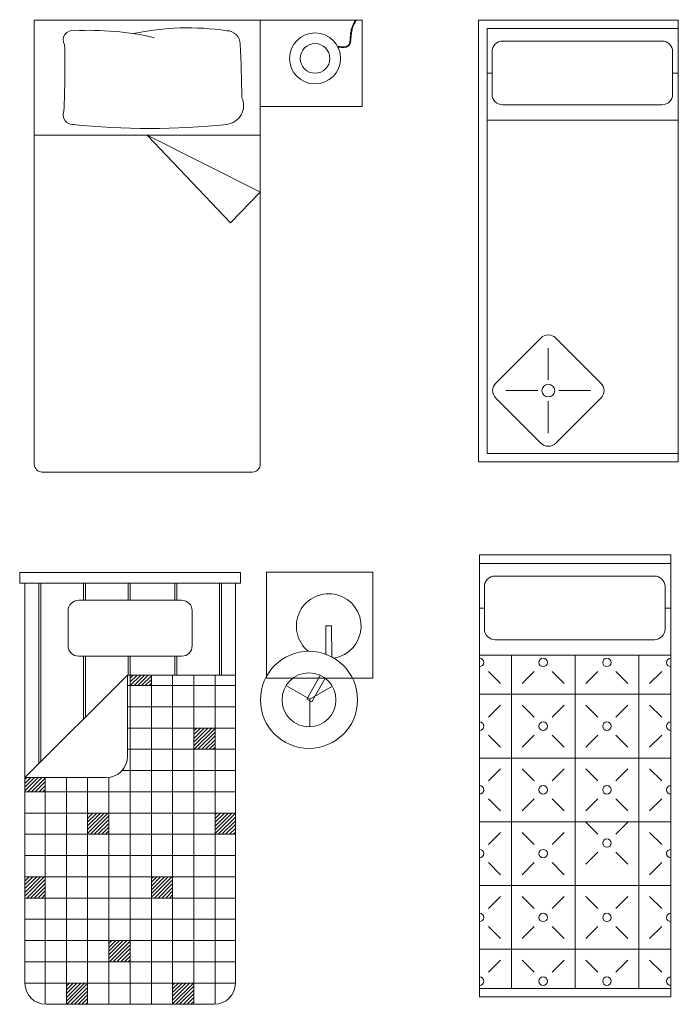
# Model space of a CAD drawing. Units: inches. Extents: x 1994 to 3075, y 3517 to 3950.
# Tile 3 of 58: x 1993.7652 to 1993.8873, y 3553.3272 to 3553.5096. Entities that reach past the tile are written whole.
import ezdxf

# ---------------------------------------------------------------- set-up
doc = ezdxf.new("R2010")
doc.units = ezdxf.units.IN
doc.layers.add('A-FURN-REFR', color=8, linetype='Continuous', lineweight=13)
doc.layers.add('A-FURN-REFR-PATT', color=8, linetype='Continuous', lineweight=13)
pattern_1 = [(45, (0, 0), (-0.0003479856204649, 0.0003479856204649), [])]
pattern_2 = [(45, (0, 0), (-0.0003479856200101, 0.0003479856200101), [])]

msp = doc.modelspace()

# ---------------------------------------------------------------- hatches: boundary and pattern name
at = {"layer": 'A-FURN-REFR-PATT'}
h = msp.add_hatch(dxfattribs=at)
h.set_pattern_fill('ANSI31', color=256, scale=0.00015500030971, style=0)
h.set_pattern_definition(pattern_2)
h.paths.add_polyline_path([(1993.785672265221, 3553.3862541341), (1993.789609273095, 3553.3862541341), (1993.789609273095, 3553.388199015989), (1993.785672265221, 3553.388199015989)])
h = msp.add_hatch(dxfattribs=at)
h.set_pattern_fill('ANSI31', color=256, scale=0.0001550003099125, style=0)
h.set_pattern_definition(pattern_1)
h.paths.add_polyline_path([(1993.797483288843, 3553.374443110477), (1993.801420296717, 3553.374443110477), (1993.801420296717, 3553.37838011835), (1993.797483288843, 3553.37838011835)])
h = msp.add_hatch(dxfattribs=at)
h.set_pattern_fill('ANSI31', color=256, scale=0.0001550003099125, style=0)
h.set_pattern_definition(pattern_1)
h.paths.add_polyline_path([(1993.766172265221, 3553.366569094728), (1993.769924233725, 3553.366569094728), (1993.769924233725, 3553.369199015988), (1993.766172265221, 3553.369199015988)])
h = msp.add_hatch(dxfattribs=at)
h.set_pattern_fill('ANSI31', color=256, scale=0.0001550003099125, style=0)
h.set_pattern_definition(pattern_1)
h.paths.add_polyline_path([(1993.777798249473, 3553.35869507898), (1993.781735257347, 3553.35869507898), (1993.781735257347, 3553.362632086854), (1993.777798249473, 3553.362632086854)])
h = msp.add_hatch(dxfattribs=at)
h.set_pattern_fill('ANSI31', color=256, scale=0.0001550003099125, style=0)
h.set_pattern_definition(pattern_1)
h.paths.add_polyline_path([(1993.801420296717, 3553.35869507898), (1993.805172265221, 3553.35869507898), (1993.805172265221, 3553.362632086854), (1993.801420296717, 3553.362632086854)])
h = msp.add_hatch(dxfattribs=at)
h.set_pattern_fill('ANSI31', color=256, scale=0.0001550003099125, style=0)
h.set_pattern_definition(pattern_1)
h.paths.add_polyline_path([(1993.766172265221, 3553.346884055358), (1993.769924233725, 3553.346884055358), (1993.769924233725, 3553.350821063232), (1993.766172265221, 3553.350821063232)])
h = msp.add_hatch(dxfattribs=at)
h.set_pattern_fill('ANSI31', color=256, scale=0.0001550003099125, style=0)
h.set_pattern_definition(pattern_1)
h.paths.add_polyline_path([(1993.789609273095, 3553.346884055358), (1993.793546280969, 3553.346884055358), (1993.793546280969, 3553.350821063232), (1993.789609273095, 3553.350821063232)])
h = msp.add_hatch(dxfattribs=at)
h.set_pattern_fill('ANSI31', color=256, scale=0.0001550003099125, style=0)
h.set_pattern_definition(pattern_1)
h.paths.add_polyline_path([(1993.781735257347, 3553.335073031736), (1993.785672265221, 3553.335073031736), (1993.785672265221, 3553.339010039611), (1993.781735257347, 3553.339010039611)])
h = msp.add_hatch(dxfattribs=at)
h.set_pattern_fill('ANSI31', color=256, scale=0.0001550003099125, style=0)
h.set_pattern_definition(pattern_1)
h.paths.add_polyline_path([(1993.773861241599, 3553.327199015988), (1993.777798249473, 3553.327199015988), (1993.777798249473, 3553.331136023862), (1993.773861241599, 3553.331136023862)])
h = msp.add_hatch(dxfattribs=at)
h.set_pattern_fill('ANSI31', color=256, scale=0.00015500030971, style=0)
h.set_pattern_definition(pattern_2)
h.paths.add_polyline_path([(1993.793546280969, 3553.327199015988), (1993.797483288843, 3553.327199015988), (1993.797483288843, 3553.331136023862), (1993.793546280969, 3553.331136023862)])

# ---------------------------------------------------------------- linework, layer by layer
at = {"layer": 'A-FURN-REFR'}
for p, q in [((1993.809793398791, 3553.509573136487), (1993.767915594969, 3553.509573136487)), ((1993.809793398791, 3553.509573136487), (1993.767915594969, 3553.509573136487)), ((1993.767915594969, 3553.509573136487), (1993.767915594969, 3553.427281987548)), ((1993.767915594969, 3553.488246379321), (1993.767915594969, 3553.509573136487)), ((1993.767915594969, 3553.509573136487), (1993.809793398791, 3553.509573136487)), ((1993.809793398791, 3553.509573136487), (1993.767915594969, 3553.509573136487)), ((1993.809793398791, 3553.509573136487), (1993.767915594969, 3553.509573136487)), ((1993.767915594969, 3553.509573136487), (1993.767915594969, 3553.427281987548)), ((1993.767915594969, 3553.488246379321), (1993.767915594969, 3553.509573136487)), ((1993.767915594969, 3553.509573136487), (1993.809793398791, 3553.509573136487)), ((1993.809793398791, 3553.509573136487), (1993.828638410511, 3553.509573136487)), ((1993.809793398791, 3553.49355757055), (1993.809793398791, 3553.509573136487)), ((1993.809793398791, 3553.509573136487), (1993.828638410511, 3553.509573136487)), ((1993.809793398791, 3553.509573136487), (1993.809793398791, 3553.488246379321)), ((1993.809793398791, 3553.509573136487), (1993.828638410511, 3553.509573136487)), ((1993.809793398791, 3553.49355757055), (1993.809793398791, 3553.509573136487)), ((1993.809793398791, 3553.509573136487), (1993.828638410511, 3553.509573136487)), ((1993.809793398791, 3553.509573136487), (1993.809793398791, 3553.488246379321)), ((1993.828638410511, 3553.509573136487), (1993.828638410511, 3553.49355757055)), ((1993.828638410511, 3553.509573136487), (1993.828638410511, 3553.49355757055)), ((1993.828638410511, 3553.509573136487), (1993.828638410511, 3553.49355757055)), ((1993.828638410511, 3553.509573136487), (1993.828638410511, 3553.49355757055)), ((1993.850243684991, 3553.427685512103), (1993.850243684991, 3553.509575275882)), ((1993.887251559007, 3553.509575275882), (1993.850243684991, 3553.509575275882)), ((1993.887251559007, 3553.427685512103), (1993.887251559007, 3553.509575275882)), ((1993.85181848814, 3553.429260315252), (1993.85181848814, 3553.508000472733)), ((1993.887251559007, 3553.508000472733), (1993.85181848814, 3553.508000472733)), ((1993.884228804072, 3553.50566943182), (1993.854701245017, 3553.50566943182)), ((1993.85273274108, 3553.503700927882), (1993.85273274108, 3553.495826912135)), ((1993.886197308009, 3553.495826912135), (1993.886197308009, 3553.503700927882)), ((1993.85181848814, 3553.499707984479), (1993.85273274108, 3553.499707984479)), ((1993.886197308009, 3553.499707984479), (1993.887251559007, 3553.499707984479)), ((1993.828638410511, 3553.49355757055), (1993.809793398791, 3553.49355757055)), ((1993.828638410511, 3553.49355757055), (1993.809793398791, 3553.49355757055)), ((1993.809793398791, 3553.427281987548), (1993.809793398791, 3553.49355757055)), ((1993.828638410511, 3553.49355757055), (1993.809793398791, 3553.49355757055)), ((1993.828638410511, 3553.49355757055), (1993.809793398791, 3553.49355757055)), ((1993.809793398791, 3553.427281987548), (1993.809793398791, 3553.49355757055)), ((1993.854701245017, 3553.493858408198), (1993.884228804072, 3553.493858408198)), ((1993.887251559007, 3553.491004982646), (1993.85181848814, 3553.491004982646)), ((1993.78885449688, 3553.488246379321), (1993.767915594969, 3553.488246379321)), ((1993.809793398791, 3553.488246379321), (1993.767915594969, 3553.488246379321)), ((1993.78885449688, 3553.488246379321), (1993.767915594969, 3553.488246379321)), ((1993.809793398791, 3553.488246379321), (1993.767915594969, 3553.488246379321)), ((1993.78885449688, 3553.488246379321), (1993.809804655327, 3553.477674335062)), ((1993.78885449688, 3553.488246379321), (1993.804276123482, 3553.472010531263)), ((1993.78885449688, 3553.488246379321), (1993.809804655327, 3553.477674335062)), ((1993.78885449688, 3553.488246379321), (1993.804276123482, 3553.472010531263)), ((1993.804276123482, 3553.472013370684), (1993.809793398791, 3553.477680015429)), ((1993.804276123482, 3553.472013370684), (1993.809793398791, 3553.477680015429)), ((1993.861770166646, 3553.450651259108), (1993.853418511751, 3553.442299604212)), ((1993.872905706508, 3553.442299604212), (1993.864554051612, 3553.450651259108)), ((1993.863162109129, 3553.448781677478), (1993.863162109129, 3553.442876165667)), ((1993.855288093381, 3553.440907661729), (1993.861193605192, 3553.440907661729)), ((1993.865130613066, 3553.440907661729), (1993.871036124877, 3553.440907661729)), ((1993.853418511751, 3553.439515719247), (1993.861770166646, 3553.431164064351)), ((1993.863162109129, 3553.438939157793), (1993.863162109129, 3553.433033645982)), ((1993.864554051612, 3553.431164064351), (1993.872905706508, 3553.439515719247)), ((1993.85181848814, 3553.429260315252), (1993.887251559007, 3553.429260315252)), ((1993.850243684991, 3553.427685512103), (1993.887251559007, 3553.427685512103)), ((1993.769380053673, 3553.425817528844), (1993.808328940087, 3553.425817528844)), ((1993.769380053673, 3553.425817528844), (1993.808328940087, 3553.425817528844)), ((1993.8504063914, 3553.328572797267), (1993.8504063914, 3553.410462561046)), ((1993.885839462266, 3553.410462561046), (1993.8504063914, 3553.410462561046)), ((1993.885839462266, 3553.328572797267), (1993.885839462266, 3553.410462561046)), ((1993.885839462266, 3553.408887757897), (1993.8504063914, 3553.408887757897)), ((1993.806140769158, 3553.407199015988), (1993.765203761284, 3553.407199015988)), ((1993.765203761284, 3553.405199015988), (1993.765203761284, 3553.407199015988)), ((1993.806140769158, 3553.405199015988), (1993.806140769158, 3553.407199015988)), ((1993.810945627877, 3553.407298841268), (1993.810945627877, 3553.387613801898)), ((1993.830630667247, 3553.407298841268), (1993.810945627877, 3553.407298841268)), ((1993.830630667247, 3553.387613801898), (1993.830630667247, 3553.407298841268)), ((1993.765203761284, 3553.405199015988), (1993.806140769158, 3553.405199015988)), ((1993.766172265221, 3553.405199015988), (1993.766172265221, 3553.331136023862)), ((1993.768743131363, 3553.405199015988), (1993.768743131363, 3553.37176988213)), ((1993.76913683215, 3553.405199015988), (1993.76913683215, 3553.372163582917)), ((1993.777010847898, 3553.405199015988), (1993.777010847898, 3553.402058913319)), ((1993.777404548685, 3553.405199015988), (1993.777404548685, 3553.402058913319)), ((1993.785278564433, 3553.405199015988), (1993.785278564433, 3553.402058913319)), ((1993.785672265221, 3553.405199015988), (1993.785672265221, 3553.402058913319)), ((1993.793939981756, 3553.405199015988), (1993.793939981756, 3553.402058913319)), ((1993.794333682544, 3553.405199015988), (1993.794333682544, 3553.402058913319)), ((1993.802207698292, 3553.405199015988), (1993.802207698292, 3553.388199015989)), ((1993.802601399079, 3553.405199015988), (1993.802601399079, 3553.388199015989)), ((1993.805172265221, 3553.331136023862), (1993.805172265221, 3553.405199015988)), ((1993.882816707332, 3553.406556716984), (1993.853289148277, 3553.406556716984)), ((1993.85132064434, 3553.404588213047), (1993.85132064434, 3553.396714197299)), ((1993.884785211269, 3553.396714197299), (1993.884785211269, 3553.404588213047)), ((1993.795203761284, 3553.402058913319), (1993.776140769158, 3553.402058913319)), ((1993.774172265221, 3553.400090409382), (1993.774172265221, 3553.393666716313)), ((1993.797172265221, 3553.393666716313), (1993.797172265221, 3553.400090409382)), ((1993.8504063914, 3553.400595269643), (1993.85132064434, 3553.400595269643)), ((1993.884785211269, 3553.400595269643), (1993.885839462266, 3553.400595269643)), ((1993.821930953234, 3553.39729858863), (1993.823003259271, 3553.397303418607)), ((1993.821954618186, 3553.392044718106), (1993.821930953234, 3553.39729858863)), ((1993.823003259271, 3553.397303418607), (1993.823029117896, 3553.391562529542)), ((1993.853289148277, 3553.394745693362), (1993.882816707332, 3553.394745693362)), ((1993.776140769158, 3553.391698212376), (1993.795203761284, 3553.391698212376)), ((1993.777010847898, 3553.391698212376), (1993.777010847898, 3553.380037598665)), ((1993.777404548685, 3553.391698212376), (1993.777404548685, 3553.380431299454)), ((1993.785278564433, 3553.391698212376), (1993.785278564433, 3553.388199015989)), ((1993.785672265221, 3553.391698212376), (1993.785672265221, 3553.388199015989)), ((1993.793939981756, 3553.391698212376), (1993.793939981756, 3553.388199015989)), ((1993.794333682544, 3553.391698212376), (1993.794333682544, 3553.388199015989)), ((1993.885839462266, 3553.39189226781), (1993.8504063914, 3553.39189226781)), ((1993.856311903211, 3553.39189226781), (1993.856311903211, 3553.330147600416)), ((1993.868122926833, 3553.39189226781), (1993.868122926833, 3553.330147600416)), ((1993.879933950455, 3553.39189226781), (1993.879933950455, 3553.330147600416)), ((1993.852076722379, 3553.388877162189), (1993.854303830351, 3553.386650054216)), ((1993.858319976071, 3553.386650054216), (1993.860547084043, 3553.388877162189)), ((1993.863887746001, 3553.388877162189), (1993.866114853974, 3553.386650054216)), ((1993.870130999692, 3553.386650054216), (1993.872358107665, 3553.388877162189)), ((1993.875698769623, 3553.388877162189), (1993.877925877595, 3553.386650054216)), ((1993.881942023315, 3553.386650054216), (1993.884169131287, 3553.388877162189)), ((1993.785172265221, 3553.388199015989), (1993.766172265221, 3553.369199015988)), ((1993.805172265221, 3553.388199015989), (1993.785172265221, 3553.388199015989)), ((1993.785172265221, 3553.373136023862), (1993.785172265221, 3553.388199015989)), ((1993.785672265221, 3553.327199015988), (1993.785672265221, 3553.388199015989)), ((1993.789609273095, 3553.327199015988), (1993.789609273095, 3553.388199015989)), ((1993.793546280969, 3553.327199015988), (1993.793546280969, 3553.388199015989)), ((1993.797483288843, 3553.327199015988), (1993.797483288843, 3553.388199015989)), ((1993.801420296717, 3553.327199015988), (1993.801420296717, 3553.388199015989)), ((1993.810945627877, 3553.387613801898), (1993.830630667247, 3553.387613801898)), ((1993.818398947116, 3553.383751910926), (1993.820873541416, 3553.388147705815)), ((1993.821807968552, 3553.387621673977), (1993.819333374252, 3553.383225879088)), ((1993.805172265221, 3553.386254134099), (1993.785172265221, 3553.386254134099)), ((1993.818978320019, 3553.383712023209), (1993.814648193, 3553.386212023209)), ((1993.818978320019, 3553.383712023209), (1993.823141804617, 3553.386115812163)), ((1993.819333374252, 3553.383225879088), (1993.818398947116, 3553.383751910926)), ((1993.818978320019, 3553.383712023209), (1993.818978320019, 3553.378712023209)), ((1993.8504063914, 3553.384641981357), (1993.885839462266, 3553.384641981357)), ((1993.805172265221, 3553.382317126224), (1993.785172265221, 3553.382317126224)), ((1993.852076722379, 3553.380406800525), (1993.854303830351, 3553.382633908498)), ((1993.858319976071, 3553.382633908498), (1993.860547084043, 3553.380406800525)), ((1993.863887746001, 3553.380406800525), (1993.866114853974, 3553.382633908498)), ((1993.870130999692, 3553.382633908498), (1993.872358107665, 3553.380406800525)), ((1993.875698769623, 3553.380406800525), (1993.877925877595, 3553.382633908498)), ((1993.881942023315, 3553.382633908498), (1993.884169131287, 3553.380406800525)), ((1993.805172265221, 3553.37838011835), (1993.785172265221, 3553.37838011835)), ((1993.852076722379, 3553.377066138567), (1993.854303830351, 3553.374839030595)), ((1993.858319976071, 3553.374839030595), (1993.860547084043, 3553.377066138567)), ((1993.863887746001, 3553.377066138567), (1993.866114853974, 3553.374839030595)), ((1993.870130999692, 3553.374839030595), (1993.872358107665, 3553.377066138567)), ((1993.875698769623, 3553.377066138567), (1993.877925877595, 3553.374839030595)), ((1993.881942023315, 3553.374839030595), (1993.884169131287, 3553.377066138567)), ((1993.805172265221, 3553.374443110477), (1993.785172265221, 3553.374443110477)), ((1993.8504063914, 3553.372830957735), (1993.885839462266, 3553.372830957735)), ((1993.805172265221, 3553.370506102603), (1993.784165026138, 3553.370506102603)), ((1993.852076722379, 3553.368595776903), (1993.854303830351, 3553.370822884875)), ((1993.858319976071, 3553.370822884875), (1993.860547084043, 3553.368595776903)), ((1993.863887746001, 3553.368595776903), (1993.866114853974, 3553.370822884875)), ((1993.870130999692, 3553.370822884875), (1993.872358107665, 3553.368595776903)), ((1993.875698769623, 3553.368595776903), (1993.877925877595, 3553.370822884875)), ((1993.881942023315, 3553.370822884875), (1993.884169131287, 3553.368595776903)), ((1993.766172265221, 3553.369199015988), (1993.781235257347, 3553.369199015988)), ((1993.769924233725, 3553.327199015988), (1993.769924233725, 3553.369199015988)), ((1993.773861241599, 3553.327199015988), (1993.773861241599, 3553.369199015988)), ((1993.777798249473, 3553.327199015988), (1993.777798249473, 3553.369199015988)), ((1993.781735257347, 3553.327199015988), (1993.781735257347, 3553.369230895055)), ((1993.805172265221, 3553.366569094728), (1993.766172265221, 3553.366569094728)), ((1993.852076722379, 3553.365255114945), (1993.854303830351, 3553.363028006972)), ((1993.858319976071, 3553.363028006972), (1993.860547084043, 3553.365255114945)), ((1993.863887746001, 3553.365255114945), (1993.866114853974, 3553.363028006972)), ((1993.870130999692, 3553.363028006972), (1993.872358107665, 3553.365255114945)), ((1993.875698769623, 3553.365255114945), (1993.877925877595, 3553.363028006972)), ((1993.881942023315, 3553.363028006972), (1993.884169131287, 3553.365255114945)), ((1993.805172265221, 3553.362632086854), (1993.766172265221, 3553.362632086854)), ((1993.8504063914, 3553.361019934113), (1993.885839462266, 3553.361019934113)), ((1993.870130999692, 3553.360969375486), (1993.872358107665, 3553.358742267513)), ((1993.875698769623, 3553.358742267513), (1993.877925877595, 3553.360969375486)), ((1993.805172265221, 3553.35869507898), (1993.766172265221, 3553.35869507898)), ((1993.852076722379, 3553.356784753281), (1993.854303830351, 3553.359011861254)), ((1993.858319976071, 3553.359011861254), (1993.860547084043, 3553.356784753281)), ((1993.863887746001, 3553.356784753281), (1993.866114853974, 3553.359011861254)), ((1993.881942023315, 3553.359011861254), (1993.884169131287, 3553.356784753281)), ((1993.805172265221, 3553.354758071107), (1993.766172265221, 3553.354758071107)), ((1993.870130999692, 3553.353174497583), (1993.872358107665, 3553.355401605556)), ((1993.875698769623, 3553.355401605556), (1993.877925877595, 3553.353174497583)), ((1993.852076722379, 3553.353444091323), (1993.854303830351, 3553.35121698335)), ((1993.858319976071, 3553.35121698335), (1993.860547084043, 3553.353444091323)), ((1993.863887746001, 3553.353444091323), (1993.866114853974, 3553.35121698335)), ((1993.881942023315, 3553.35121698335), (1993.884169131287, 3553.353444091323)), ((1993.805172265221, 3553.350821063232), (1993.766172265221, 3553.350821063232)), ((1993.8504063914, 3553.349208910491), (1993.885839462266, 3553.349208910491)), ((1993.805172265221, 3553.346884055358), (1993.766172265221, 3553.346884055358)), ((1993.852076722379, 3553.344973729659), (1993.854303830351, 3553.347200837631)), ((1993.858319976071, 3553.347200837631), (1993.860547084043, 3553.344973729659)), ((1993.863887746001, 3553.344973729659), (1993.866114853974, 3553.347200837631)), ((1993.870130999692, 3553.347200837631), (1993.872358107665, 3553.344973729659)), ((1993.875698769623, 3553.344973729659), (1993.877925877595, 3553.347200837631)), ((1993.881942023315, 3553.347200837631), (1993.884169131287, 3553.344973729659)), ((1993.805172265221, 3553.342947047485), (1993.766172265221, 3553.342947047485)), ((1993.852076722379, 3553.341633067701), (1993.854303830351, 3553.339405959729)), ((1993.858319976071, 3553.339405959729), (1993.860547084043, 3553.341633067701)), ((1993.863887746001, 3553.341633067701), (1993.866114853974, 3553.339405959729)), ((1993.870130999692, 3553.339405959729), (1993.872358107665, 3553.341633067701)), ((1993.875698769623, 3553.341633067701), (1993.877925877595, 3553.339405959729)), ((1993.881942023315, 3553.339405959729), (1993.884169131287, 3553.341633067701)), ((1993.805172265221, 3553.339010039611), (1993.766172265221, 3553.339010039611)), ((1993.8504063914, 3553.337397886869), (1993.885839462266, 3553.337397886869)), ((1993.805172265221, 3553.335073031736), (1993.766172265221, 3553.335073031736)), ((1993.852076722379, 3553.333162706036), (1993.854303830351, 3553.335389814009)), ((1993.858319976071, 3553.335389814009), (1993.860547084043, 3553.333162706036)), ((1993.863887746001, 3553.333162706036), (1993.866114853974, 3553.335389814009)), ((1993.870130999692, 3553.335389814009), (1993.872358107665, 3553.333162706036)), ((1993.875698769623, 3553.333162706036), (1993.877925877595, 3553.335389814009)), ((1993.881942023315, 3553.335389814009), (1993.884169131287, 3553.333162706036)), ((1993.805172265221, 3553.331136023862), (1993.766172265221, 3553.331136023862)), ((1993.8504063914, 3553.330147600416), (1993.885839462266, 3553.330147600416)), ((1993.8504063914, 3553.328572797267), (1993.885839462266, 3553.328572797267)), ((1993.770109273095, 3553.327199015988), (1993.801235257347, 3553.327199015988))]:
    msp.add_line(p, q, dxfattribs=at)
for centre, radius in [((1993.819937102994, 3553.502455661661), 0.004728775123852), ((1993.819937102994, 3553.502455661661), 0.004728775123852), ((1993.819937102994, 3553.502455661661), 0.0027401859108547), ((1993.819937102994, 3553.502455661661), 0.0027401859108547), ((1993.863162109129, 3553.440907661729), 0.0011811023622047), ((1993.818814975856, 3553.383610108095), 0.009), ((1993.862217415022, 3553.390547493168), 0.0007874015748031), ((1993.874028438644, 3553.390547493168), 0.0007874015748031), ((1993.818814975856, 3553.383610108095), 0.005), ((1993.862217415022, 3553.378736469546), 0.0007874015748031), ((1993.874028438644, 3553.378736469546), 0.0007874015748031), ((1993.862217415022, 3553.366925445924), 0.0007874015748031), ((1993.874028438644, 3553.366925445924), 0.0007874015748031), ((1993.874028438644, 3553.357071936534), 0.0007874015748031), ((1993.862217415022, 3553.355114422302), 0.0007874015748031), ((1993.862217415022, 3553.34330339868), 0.0007874015748031), ((1993.874028438644, 3553.34330339868), 0.0007874015748031), ((1993.862217415022, 3553.331492375058), 0.0007874015748031), ((1993.874028438644, 3553.331492375058), 0.0007874015748031)]:
    msp.add_circle(centre, radius, dxfattribs=at)
for centre, radius, start, end in [((1993.774987817538, 3553.505899838229), 0.0017217387327707, 78.72778623498706, 211.6094986857782), ((1993.774987817538, 3553.505899838229), 0.0017217387327707, 78.72778623498706, 211.6094986857782), ((1993.778177087261, 3553.454028661814), 0.0536356196908511, 77.05638185161688, 93.04883220562752), ((1993.778177087261, 3553.454028661814), 0.0536356196908511, 77.05638185161688, 93.04883220562752), ((1993.796412637469, 3553.459797290203), 0.0483256070365364, 81.47022635647696, 102.1032641982298), ((1993.796412637469, 3553.459797290203), 0.0483256070365364, 81.47022635647696, 102.1032641982298), ((1993.803580452496, 3553.505110780277), 0.0024775836026722, 0, 90), ((1993.803580452496, 3553.505110780277), 0.0024775836026722, 0, 90), ((1993.854701245017, 3553.503700927882), 0.0019685039370078, 90, 180), ((1993.884228804072, 3553.503700927882), 0.0019685039370078, 0, 90), ((1993.59619628872, 3553.500652075388), 0.1773784605747312, 357.4333292641344, 1.403751564921032), ((1993.59619628872, 3553.500652075388), 0.1773784605747312, 357.4333292641344, 1.403751564921032), ((1993.511365803193, 3553.490522296764), 0.2950531070603349, 0.9125644663952034, 2.834064295864955), ((1993.511365803193, 3553.490522296764), 0.2950531070603349, 0.9125644663952034, 2.834064295864955), ((1993.803146714828, 3553.493755870891), 0.0035513056944607, 277.015318444972, 24.37436785420747), ((1993.803146714828, 3553.493755870891), 0.0035513056944607, 277.015318444972, 24.37436785420747), ((1993.854701245017, 3553.495826912135), 0.0019685039370081, 180, 270), ((1993.884228804072, 3553.495826912135), 0.0019685039370081, 270, 0), ((1993.775025526006, 3553.491987270096), 0.0017813637547286, 156.1084115545774, 279.6575795622506), ((1993.775025526006, 3553.491987270096), 0.0017813637547286, 156.1084115545774, 279.6575795622506), ((1993.789181602352, 3553.627517539036), 0.1380394109326758, 264.1139139330622, 275.9873971424126), ((1993.789181602352, 3553.627517539036), 0.1380394109326758, 264.1139139330622, 275.9873971424126), ((1993.863162109129, 3553.449259316626), 0.0019685039370078, 45, 135), ((1993.854810454233, 3553.440907661729), 0.0019685039370079, 135, 225), ((1993.871513764025, 3553.440907661729), 0.0019685039370079, 315, 45), ((1993.863162109129, 3553.432556006834), 0.0019685039370079, 225, 315), ((1993.769380053673, 3553.427281987548), 0.0014644587043272, 180, 270), ((1993.769380053673, 3553.427281987548), 0.0014644587043272, 180, 270), ((1993.808328940087, 3553.427281987548), 0.0014644587043272, 270, 0), ((1993.808328940087, 3553.427281987548), 0.0014644587043272, 270, 0), ((1993.853289148277, 3553.404588213047), 0.0019685039370078, 90, 180), ((1993.882816707332, 3553.404588213047), 0.0019685039370078, 0, 90), ((1993.822475229895, 3553.397270362133), 0.006, 279.0280450997825, 230.9719549002995), ((1993.776140769158, 3553.400090409382), 0.0019685039370061, 90, 180), ((1993.795203761284, 3553.400090409382), 0.0019685039370072, 0, 90), ((1993.853289148277, 3553.396714197299), 0.0019685039370081, 180, 270), ((1993.882816707332, 3553.396714197299), 0.0019685039370081, 270, 0), ((1993.776140769158, 3553.393666716313), 0.0019685039370083, 180, 270), ((1993.795203761284, 3553.393666716313), 0.0019685039370083, 270, 0), ((1993.8504063914, 3553.390547493168), 0.0007874015748031, 270, 90), ((1993.885839462266, 3553.390547493168), 0.0007874015748031, 90, 270), ((1993.8504063914, 3553.378736469546), 0.0007874015748031, 270, 90), ((1993.885839462266, 3553.378736469546), 0.0007874015748031, 90, 270), ((1993.781235257347, 3553.373136023862), 0.0039370078740144, 270, 0), ((1993.8504063914, 3553.366925445924), 0.0007874015748031, 270, 90), ((1993.885839462266, 3553.366925445924), 0.0007874015748031, 90, 270), ((1993.8504063914, 3553.355114422302), 0.0007874015748031, 270, 90), ((1993.885839462266, 3553.355114422302), 0.0007874015748031, 90, 270), ((1993.8504063914, 3553.34330339868), 0.0007874015748031, 270, 90), ((1993.885839462266, 3553.34330339868), 0.0007874015748031, 90, 270), ((1993.8504063914, 3553.331492375058), 0.0007874015748031, 270, 90), ((1993.885839462266, 3553.331492375058), 0.0007874015748031, 90, 270), ((1993.770109273095, 3553.331136023862), 0.0039370078740155, 180, 270), ((1993.801235257347, 3553.331136023862), 0.0039370078740166, 270, 0)]:
    msp.add_arc(centre, radius, start, end, dxfattribs=at)
for points, knots in [([(1993.824177946201, 3553.504547685339), (1993.824971585506, 3553.504474400106), (1993.826725153512, 3553.504325811513), (1993.82643117435, 3553.50738811441), (1993.82717809387, 3553.508830991155), (1993.827574916962, 3553.509573136487)], [0, 0, 0, 0, 0.0019919301600581, 0.0044204930031509, 0.0070212840221272, 0.0070212840221272, 0.0070212840221272, 0.0070212840221272]), ([(1993.824177946201, 3553.504547685339), (1993.824971585506, 3553.504474400106), (1993.826725153512, 3553.504325811513), (1993.82643117435, 3553.50738811441), (1993.82717809387, 3553.508830991155), (1993.827574916962, 3553.509573136487)], [0, 0, 0, 0, 0.0019919301600581, 0.0044204930031509, 0.0070212840221272, 0.0070212840221272, 0.0070212840221272, 0.0070212840221272]), ([(1993.824189597779, 3553.504673865603), (1993.824314014164, 3553.504662376903), (1993.824437937851, 3553.504650936942), (1993.824803510088, 3553.504621615954), (1993.8250390861, 3553.504608843931), (1993.825425334499, 3553.504620031528), (1993.825583507578, 3553.504637555722), (1993.825865461475, 3553.50470914596), (1993.825984414765, 3553.504765314885), (1993.8261485078, 3553.504908351171), (1993.826207876676, 3553.504992451086), (1993.826305031139, 3553.505201194998), (1993.82634194283, 3553.505325217223), (1993.826425686936, 3553.505741490427), (1993.826444320893, 3553.506075609908), (1993.826477761296, 3553.506645383253), (1993.826491915599, 3553.506875653857), (1993.82656018031, 3553.507427868108), (1993.826632437549, 3553.507734428252), (1993.826818921189, 3553.50831097189), (1993.826933004782, 3553.508581901063), (1993.827185626783, 3553.509113916526), (1993.827324903756, 3553.50937429669), (1993.827463171123, 3553.509632886683)], [0, 0, 0, 0, 0.7456664768345322, 0.7456664768345322, 2.236999430503596, 2.236999430503596, 3.442388313778277, 3.442388313778277, 4.740874518937371, 4.740874518937371, 5.813128485196044, 5.813128485196044, 6.885382451454717, 6.885382451454717, 9.044396613967223, 9.044396613967223, 10.46205112301665, 10.46205112301665, 12.54798424783743, 12.54798424783743, 14.63391737265821, 14.63391737265821, 16.79785288112622, 16.79785288112622, 16.79785288112622, 16.79785288112622]), ([(1993.824189597779, 3553.504673865603), (1993.824314014164, 3553.504662376903), (1993.824437937851, 3553.504650936942), (1993.824803510088, 3553.504621615954), (1993.8250390861, 3553.504608843931), (1993.825425334499, 3553.504620031528), (1993.825583507578, 3553.504637555722), (1993.825865461475, 3553.50470914596), (1993.825984414765, 3553.504765314885), (1993.8261485078, 3553.504908351171), (1993.826207876676, 3553.504992451086), (1993.826305031139, 3553.505201194998), (1993.82634194283, 3553.505325217223), (1993.826425686936, 3553.505741490427), (1993.826444320893, 3553.506075609908), (1993.826477761296, 3553.506645383253), (1993.826491915599, 3553.506875653857), (1993.82656018031, 3553.507427868108), (1993.826632437549, 3553.507734428252), (1993.826818921189, 3553.50831097189), (1993.826933004782, 3553.508581901063), (1993.827185626783, 3553.509113916526), (1993.827324903756, 3553.50937429669), (1993.827463171123, 3553.509632886683)], [0, 0, 0, 0, 0.7456664768345322, 0.7456664768345322, 2.236999430503596, 2.236999430503596, 3.442388313778277, 3.442388313778277, 4.740874518937371, 4.740874518937371, 5.813128485196044, 5.813128485196044, 6.885382451454717, 6.885382451454717, 9.044396613967223, 9.044396613967223, 10.46205112301665, 10.46205112301665, 12.54798424783743, 12.54798424783743, 14.63391737265821, 14.63391737265821, 16.79785288112622, 16.79785288112622, 16.79785288112622, 16.79785288112622])]:
    msp.add_open_spline(points, degree=3, knots=knots, dxfattribs=at)

doc.saveas('drawing.dxf')
